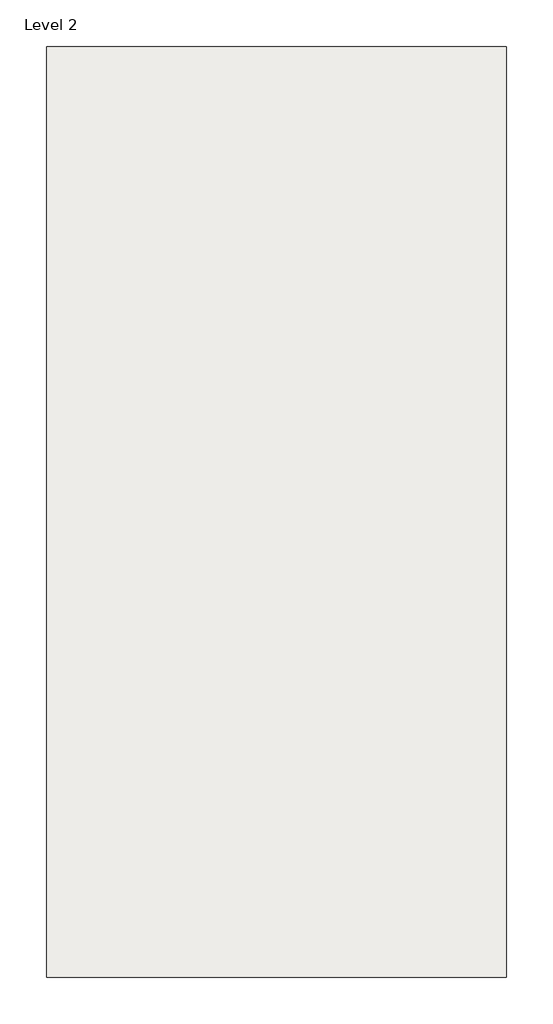
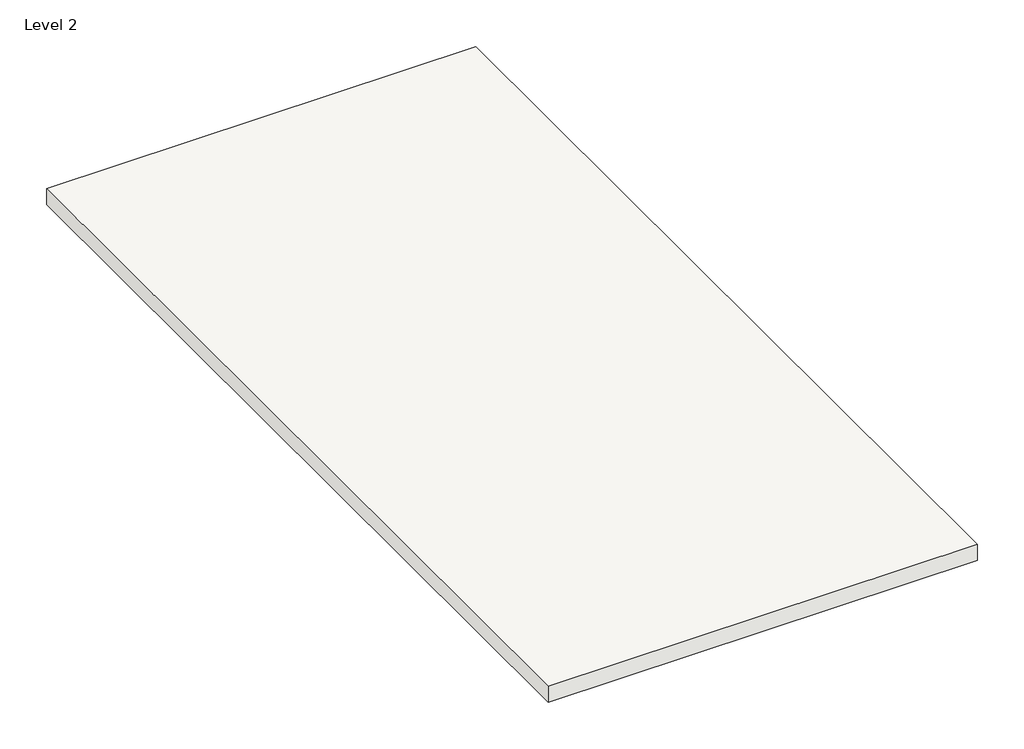
# One storey: 1 roof.
"""IFC4 building model written with IfcOpenShell, lengths in millimetres."""

from ifc_helpers import new_model, si_unit, frame, origin, place, context, project, spatial, polyline, outline, extrude, element, save

model = new_model("IFC4")

# Units and contexts
model_context = context("Model", 3, world=origin())
ifc_project = project(units=[si_unit("LENGTHUNIT", "METRE", prefix="MILLI")], contexts=[model_context])

# Site, building, storey
site = spatial("IfcSite", under=ifc_project)
building = spatial("IfcBuilding", under=site)
storey = spatial("IfcBuildingStorey", under=building, Name="Level 2", Elevation=3048.0)

# Roof
placement = place(None, origin())
element("IfcRoof", 1, ObjectType="Generic - 12\"", at=placement, inside=storey, context=model_context, shape_type="SweptSolid", body=[
    extrude(outline(polyline([(-16280.7905738, 11195.7768478), (-8444.8905738, 11195.7768478), (-8444.8905738, -4653.8231522), (-16280.7905738, -4653.8231522), (-16280.7905738, 11195.7768478)])), frame((0.0, 0.0, 3048.0), z_axis=(0.0, 0.0, 1.0), x_axis=(1.0, 0.0, 0.0)), (0.0, 0.0, 1.0), 304.8),
])

save(model, "model.ifc")

# Revit data of these elements
# Type "Generic - 12\""
#   Assembly Code = "B1020"
#   Layers, outside or top first: 1' - 0" no material (function 1)
# Element 1 (IfcRoof, "Generic - 12\"")
#   built-in parameter 1001705 = 11 (stored number, unit not read)
#   built-in parameter 1001710 = 33615
#   Phase Created = New Construction
#   Materials on its faces: "Default Roof"
# Materials
#   "Default Roof": colour RGB 88 101 114, transparency 0
